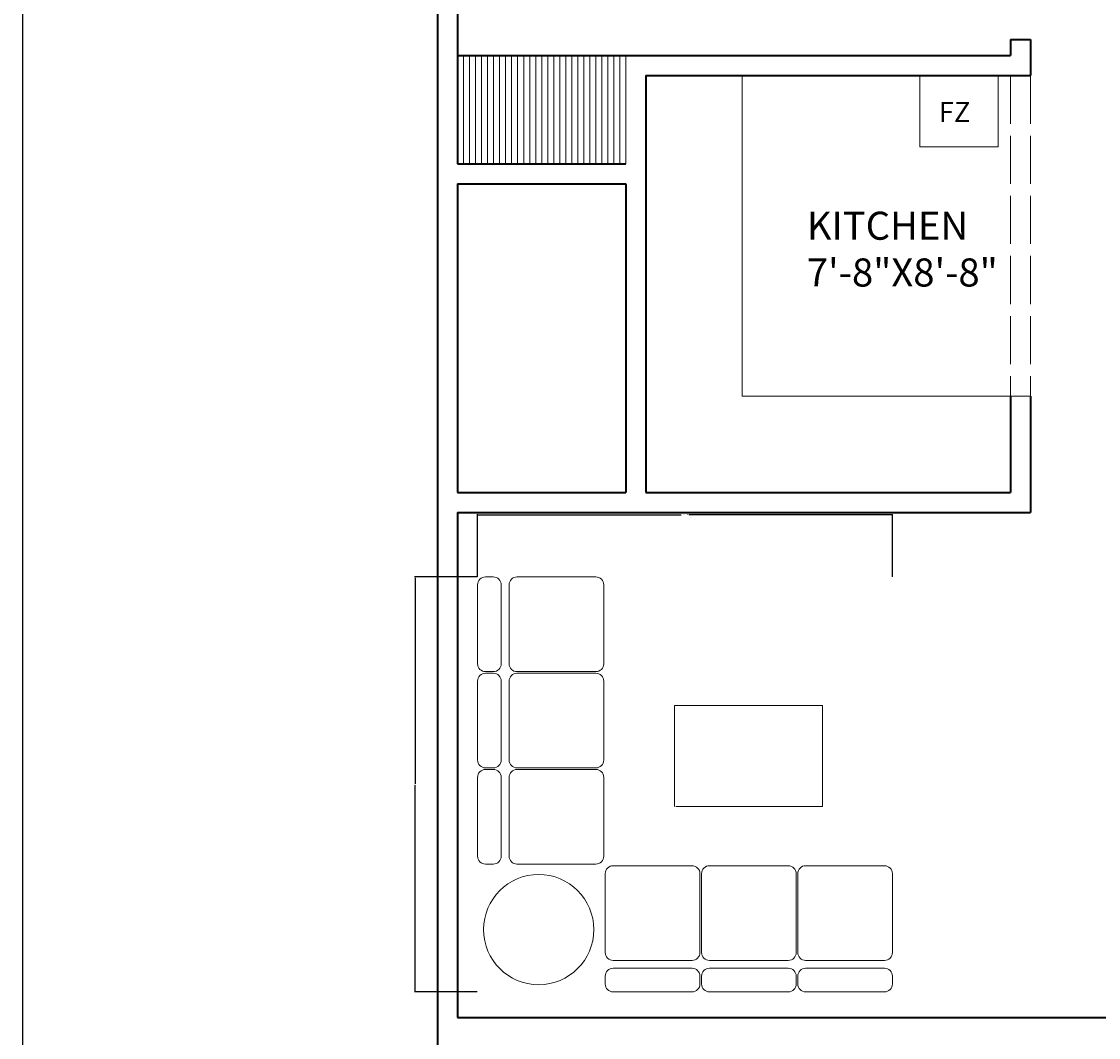
# Model space of a CAD drawing. Units: inches. Extents: x 3731 to 4318, y 1310 to 2388.
# Tile 33 of 57: x 3731 to 4000, y 1938 to 2192. Entities that reach past the tile are written whole.
import ezdxf

# ---------------------------------------------------------------- set-up
doc = ezdxf.new("R2010")
doc.units = ezdxf.units.IN
doc.linetypes.add('ACAD_ISO02W100', pattern=[15, 12, -3])
for name, color, linetype, lineweight in [('A-ANNO-DIMS', 2, 'Continuous', 18), ('A-ANNO-TEXT', 7, 'Continuous', 18), ('A-AREA-IDEN', 7, 'Continuous', 18), ('A-EQPM', 8, 'Continuous', 18), ('A-FLOR-CASE', 8, 'Continuous', 18), ('A-FLOR-PATT', 252, 'Continuous', 13), ('A-FURN', 8, 'Continuous', 13), ('A-WALL', 7, 'Continuous', 35), ('A-WALL-OVHD', 7, 'ACAD_ISO02W100', 18)]:
    doc.layers.add(name, color=color, linetype=linetype, lineweight=lineweight)
doc.styles.get("Standard").update_dxf_attribs({"font": 'arial.ttf'})
doc.dimstyles.get("Standard").update_dxf_attribs({"dimtxt": 0.18, "dimasz": 0.18, "dimexe": 0.18, "dimexo": 0.0625, "dimgap": 0.09, "dimtad": 0, "dimtih": 1, "dimtoh": 1, "dimdec": 4, "dimzin": 0, "dimdsep": 46, "dimtxsty": 'Standard', "dimcen": 0.09, "dimadec": 0, "dimazin": 0, "dimtfac": 1, "dimtdec": 4, "dimtofl": 0, "dimtmove": 0, "dimatfit": 3, "dimfxl": 1, "dimtolj": 1, "dimtzin": 0, "dimarcsym": 0})

# ---------------------------------------------------------------- blocks, each defined once
blk = doc.blocks.new('*U3')
blk.add_line((0, 0), (0, 27))
blk = doc.blocks.new('*U4')
at = {"layer": 'A-FLOR-PATT', "color": 0, "linetype": 'ByBlock', "lineweight": -2, "transparency": 16777216, "rotation": 180}
for p in [(3840.21, 2183.38), (3841.71, 2183.38), (3843.21, 2183.38), (3844.71, 2183.38), (3846.21, 2183.38), (3847.71, 2183.38), (3849.21, 2183.38), (3850.71, 2183.38), (3852.21, 2183.38), (3853.71, 2183.38), (3855.21, 2183.38), (3856.71, 2183.38), (3858.21, 2183.38), (3859.71, 2183.38), (3861.21, 2183.38), (3862.71, 2183.38), (3864.21, 2183.38), (3865.71, 2183.38), (3867.21, 2183.38), (3868.71, 2183.38), (3870.21, 2183.38), (3871.71, 2183.38), (3873.21, 2183.38), (3874.71, 2183.38), (3876.21, 2183.38), (3877.71, 2183.38), (3879.21, 2183.38), (3880.71, 2183.38), (3882.21, 2183.38)]:
    blk.add_blockref('*U3', p, dxfattribs=at)
blk = doc.blocks.new('A$C753D6792')
at = {"linetype": 'ByBlock'}
for p, q in [((50, 2630), (550, 2630)), ((660, 2630), (1160, 2630)), ((1270, 2630), (1770, 2630)), ((0, 2530), (0, 2580)), ((600, 2580), (600, 2530)), ((610, 2530), (610, 2580)), ((1210, 2580), (1210, 2530)), ((1220, 2530), (1220, 2580)), ((1820, 2580), (1820, 2530)), ((550, 2480), (50, 2480)), ((1160, 2480), (660, 2480)), ((1770, 2480), (1270, 2480)), ((550, 2430), (50, 2430)), ((1160, 2430), (660, 2430)), ((1770, 2430), (1270, 2430)), ((0, 1880), (0, 2380)), ((600, 2380), (600, 1880)), ((610, 1880), (610, 2380)), ((1210, 2380), (1210, 1880)), ((1220, 1880), (1220, 2380)), ((1820, 1880), (1820, 2380)), ((50, 1830), (427.2, 1830)), ((386.5, 1830), (550, 1830)), ((660, 1830), (1037.2, 1830)), ((996.5, 1830), (1160, 1830)), ((1270, 1830), (1647.2, 1830)), ((1606.5, 1830), (1770, 1830)), ((1880, 1820), (2380, 1820)), ((2530, 1820), (2580, 1820)), ((1830, 1770), (1830, 1392.8)), ((2430, 1270), (2430, 1770)), ((2480, 1270), (2480, 1770)), ((2630, 1770), (2630, 1270)), ((442.3, 815), (442.3, 1455)), ((442.3, 1455), (1372.3, 1455)), ((1382.3, 1455), (1382.3, 815)), ((1830, 1433.5), (1830, 1270)), ((2380, 1220), (1880, 1220)), ((1880, 1210), (2380, 1210)), ((2580, 1220), (2530, 1220)), ((2530, 1210), (2580, 1210)), ((1830, 1160), (1830, 782.8)), ((2430, 660), (2430, 1160)), ((2480, 660), (2480, 1160)), ((2630, 1160), (2630, 660)), ((1830, 823.5), (1830, 660)), ((1382.3, 815), (442.3, 815)), ((1830, 550), (1830, 172.8)), ((2380, 610), (1880, 610)), ((1880, 600), (2380, 600)), ((2430, 50), (2430, 550)), ((2480, 50), (2480, 550)), ((2580, 610), (2530, 610)), ((2530, 600), (2580, 600)), ((2630, 550), (2630, 50)), ((1830, 213.5), (1830, 50)), ((2380, 0), (1880, 0)), ((2580, 0), (2530, 0))]:
    blk.add_line(p, q, dxfattribs=at)
blk.add_circle((2242.3, 2235), 349.3, dxfattribs=at)
for centre, start, end in [((50, 2580), 90, 180), ((550, 2580), 0, 90), ((550, 2580), 0, 90), ((660, 2580), 90, 180), ((1160, 2580), 0, 90), ((1160, 2580), 0, 90), ((1270, 2580), 90, 180), ((1770, 2580), 0, 90), ((1770, 2580), 0, 90), ((50, 2530), 180, 270), ((550, 2530), 270, 0), ((550, 2530), 270, 0), ((660, 2530), 180, 270), ((1160, 2530), 270, 0), ((1160, 2530), 270, 0), ((1270, 2530), 180, 270), ((1770, 2530), 270, 0), ((1770, 2530), 270, 0), ((50, 2380), 90, 180), ((550, 2380), 0, 90), ((550, 2380), 0, 90), ((660, 2380), 90, 180), ((1160, 2380), 0, 90), ((1160, 2380), 0, 90), ((1270, 2380), 90, 180), ((1770, 2380), 0, 90), ((1770, 2380), 0, 90), ((50, 1880), 180, 270), ((550, 1880), 270, 0), ((660, 1880), 180, 270), ((1160, 1880), 270, 0), ((1270, 1880), 180, 270), ((1770, 1880), 270, 0), ((1880, 1770), 90, 180), ((2380, 1770), 0, 90), ((2530, 1770), 90, 180), ((2580, 1770), 0, 90), ((1880, 1270), 180, 270), ((2380, 1270), 270, 0), ((2380, 1270), 270, 0), ((2530, 1270), 180, 270), ((2530, 1270), 180, 270), ((2580, 1270), 270, 0), ((2580, 1270), 270, 0), ((1880, 1160), 90, 180), ((2380, 1160), 0, 90), ((2530, 1160), 90, 180), ((2580, 1160), 0, 90), ((1880, 660), 180, 270), ((2380, 660), 270, 0), ((2380, 660), 270, 0), ((2530, 660), 180, 270), ((2530, 660), 180, 270), ((2580, 660), 270, 0), ((2580, 660), 270, 0), ((1880, 550), 90, 180), ((2380, 550), 0, 90), ((2530, 550), 90, 180), ((2580, 550), 0, 90), ((1880, 50), 180, 270), ((2380, 50), 270, 0), ((2380, 50), 270, 0), ((2530, 50), 180, 270), ((2530, 50), 180, 270), ((2580, 50), 270, 0), ((2580, 50), 270, 0)]:
    blk.add_arc(centre, 50, start, end, dxfattribs=at)
blk = doc.blocks.new('*D20')
at = {"layer": 'A-ANNO-DIMS', "color": 0, "lineweight": -2, "transparency": 16777216}
for p, q in [((3845.19, 2053.34), (3845.19, 2068.99)), ((3845.37, 2068.81), (3896.02, 2068.81)), ((3948.56, 2068.81), (3897.91, 2068.81)), ((3948.74, 2053.34), (3948.74, 2068.99))]:
    blk.add_line(p, q, dxfattribs=at)
at = {"layer": 'A-ANNO-DIMS', "color": 0, "transparency": 16777216}
for points in [[(3845.37, 2068.84), (3845.37, 2068.78), (3845.19, 2068.81)], [(3948.56, 2068.84), (3948.56, 2068.78), (3948.74, 2068.81)]]:
    blk.add_solid(points, dxfattribs=at)
at = {"layer": 'Defpoints', "color": 0, "transparency": 16777216}
for p in [(3845.19, 2068.81), (3845.19, 2053.28), (3948.74, 2053.28)]:
    blk.add_point(p, dxfattribs=at)
at = {"layer": 'A-ANNO-DIMS', "color": 0, "transparency": 16777216, "insert": (3896.97, 2068.81), "char_height": 0.18, "attachment_point": 5}
blk.add_mtext('\\A1;SOFA SET 104', dxfattribs=at)
blk = doc.blocks.new('*D21')
at = {"layer": 'A-ANNO-DIMS', "color": 0, "lineweight": -2, "transparency": 16777216}
for p, q in [((3845.13, 2053.28), (3829.48, 2053.28)), ((3829.66, 2053.1), (3829.66, 2001.69)), ((3829.66, 1949.91), (3829.66, 2001.32)), ((3845.13, 1949.73), (3829.48, 1949.73))]:
    blk.add_line(p, q, dxfattribs=at)
at = {"layer": 'A-ANNO-DIMS', "color": 0, "transparency": 16777216}
for points in [[(3829.63, 2053.1), (3829.69, 2053.1), (3829.66, 2053.28)], [(3829.63, 1949.91), (3829.69, 1949.91), (3829.66, 1949.73)]]:
    blk.add_solid(points, dxfattribs=at)
at = {"layer": 'Defpoints', "color": 0, "transparency": 16777216}
for p in [(3845.19, 2053.28), (3829.66, 1949.73), (3845.19, 1949.73)]:
    blk.add_point(p, dxfattribs=at)
at = {"layer": 'A-ANNO-DIMS', "color": 0, "transparency": 16777216, "insert": (3829.66, 2001.5), "char_height": 0.18, "attachment_point": 5}
blk.add_mtext('\\A1;104', dxfattribs=at)
blk = doc.blocks.new('*D33')
at = {"layer": 'A-ANNO-DIMS', "color": 0, "lineweight": -2, "transparency": 16777216}
for p, q in [((3835.15, 2338.38), (3731.41, 2338.38)), ((3731.59, 2338.2), (3731.59, 1849.06)), ((3731.59, 1359.56), (3731.59, 1848.7)), ((3835.15, 1359.38), (3731.41, 1359.38))]:
    blk.add_line(p, q, dxfattribs=at)
at = {"layer": 'A-ANNO-DIMS', "color": 0, "transparency": 16777216}
for points in [[(3731.56, 2338.2), (3731.62, 2338.2), (3731.59, 2338.38)], [(3731.56, 1359.56), (3731.62, 1359.56), (3731.59, 1359.38)]]:
    blk.add_solid(points, dxfattribs=at)
at = {"layer": 'Defpoints', "color": 0, "transparency": 16777216}
for p in [(3731.59, 2338.38), (3835.21, 2338.38), (3835.21, 1359.38)]:
    blk.add_point(p, dxfattribs=at)
at = {"layer": 'A-ANNO-DIMS', "color": 0, "transparency": 16777216, "insert": (3731.59, 1848.88), "char_height": 0.18, "attachment_point": 5}
blk.add_mtext('\\A1;979', dxfattribs=at)

msp = doc.modelspace()

# ---------------------------------------------------------------- linework, layer by layer
at = {"layer": 'A-EQPM'}
msp.add_lwpolyline([(3955.62, 2178.38), (3975.16, 2178.38), (3975.16, 2160.61), (3955.62, 2160.61)], close=True, dxfattribs=at)
at = {"layer": 'A-FLOR-CASE'}
for p, q in [((3911.21, 2178.38), (3911.21, 2098.38)), ((3911.21, 2098.38), (3983.21, 2098.38))]:
    msp.add_line(p, q, dxfattribs=at)
at = {"layer": 'A-WALL'}
for p, q in [((3835.21, 2338.38), (3835.21, 1359.38)), ((3840.21, 2333.38), (3840.21, 2156.38)), ((3978.21, 2187.38), (3983.21, 2187.38)), ((3978.21, 2187.38), (3978.21, 2183.38)), ((3983.21, 2187.38), (3983.21, 2178.38)), ((3840.21, 2183.38), (3882.21, 2183.38)), ((3882.21, 2183.38), (3978.21, 2183.38)), ((3887.21, 2178.38), (3887.21, 2074.38)), ((3887.21, 2178.38), (3983.21, 2178.38)), ((3840.21, 2156.38), (3882.21, 2156.38)), ((3840.21, 2151.38), (3882.21, 2151.38)), ((3840.21, 2151.38), (3840.21, 2074.38)), ((3882.21, 2151.38), (3882.21, 2074.38)), ((3978.21, 2098.38), (3978.21, 2074.38)), ((3983.21, 2098.38), (3983.21, 2069.38)), ((3840.21, 2074.38), (3882.21, 2074.38)), ((3887.21, 2074.38), (3978.21, 2074.38)), ((3840.21, 2069.38), (3983.21, 2069.38)), ((3840.21, 2069.38), (3840.21, 1943.38)), ((3840.21, 1943.38), (4055.21, 1943.38))]:
    msp.add_line(p, q, dxfattribs=at)
at = {"layer": 'A-WALL-OVHD'}
for p, q in [((3978.21, 2178.38), (3978.21, 2098.38)), ((3983.21, 2178.38), (3983.21, 2098.38))]:
    msp.add_line(p, q, dxfattribs=at)

# ---------------------------------------------------------------- block references
at = {"layer": 'A-FLOR-PATT'}
msp.add_blockref('*U4', (0, 0), dxfattribs=at)
at = {"layer": 'A-FURN', "xscale": 0.0393700787401575, "yscale": 0.0393700787401575, "zscale": 0.0393700787401575, "rotation": 180}
msp.add_blockref('A$C753D6792', (3948.74, 2053.28), dxfattribs=at)

# ---------------------------------------------------------------- texts
at = {"layer": 'A-ANNO-TEXT', "insert": (3960.33, 2171.8), "char_height": 5, "attachment_point": 1}
msp.add_mtext_dynamic_manual_height_columns('FZ', width=11.089, gutter_width=12.5, heights=[0], dxfattribs=at)
at = {"layer": 'A-AREA-IDEN', "insert": (3927.38, 2144.43), "char_height": 7, "attachment_point": 1}
msp.add_mtext_dynamic_manual_height_columns('KITCHEN\\P7\'-8"X8\'-8"', width=24.0878, gutter_width=12.5, heights=[0], dxfattribs=at)

# ---------------------------------------------------------------- dimensions: what is measured, and where the dimension line sits
at = {"layer": 'A-ANNO-DIMS'}
for base, p1, p2, angle, picture, middle in [((3731.59, 2338.38), (3835.21, 1359.38), (3835.21, 2338.38), 90, '*D33', (3731.59, 1848.88)), ((3829.66, 1949.73), (3845.19, 2053.28), (3845.19, 1949.73), 270, '*D21', (3829.66, 2001.5))]:
    dim = msp.add_linear_dim(base=base, p1=p1, p2=p2, angle=angle, dimstyle='Standard', override={"dimdec": 0, "dimlfac": 1, "dimrnd": 0, "dimzin": 0, "dimdsep": 46, "dimlunit": 2}, dxfattribs=at)
    dim.commit()
    dim.dimension.update_dxf_attribs({"geometry": picture, "text_midpoint": middle})
dim = msp.add_linear_dim(base=(3845.19, 2068.81), p1=(3948.74, 2053.28), p2=(3845.19, 2053.28), angle=180, text='SOFA SET <>', dimstyle='Standard', override={"dimdec": 0, "dimlfac": 1, "dimrnd": 0, "dimzin": 0, "dimdsep": 46, "dimlunit": 2}, dxfattribs=at)
dim.commit()
dim.dimension.update_dxf_attribs({"geometry": '*D20', "text_midpoint": (3896.97, 2068.81)})

doc.saveas('drawing.dxf')
